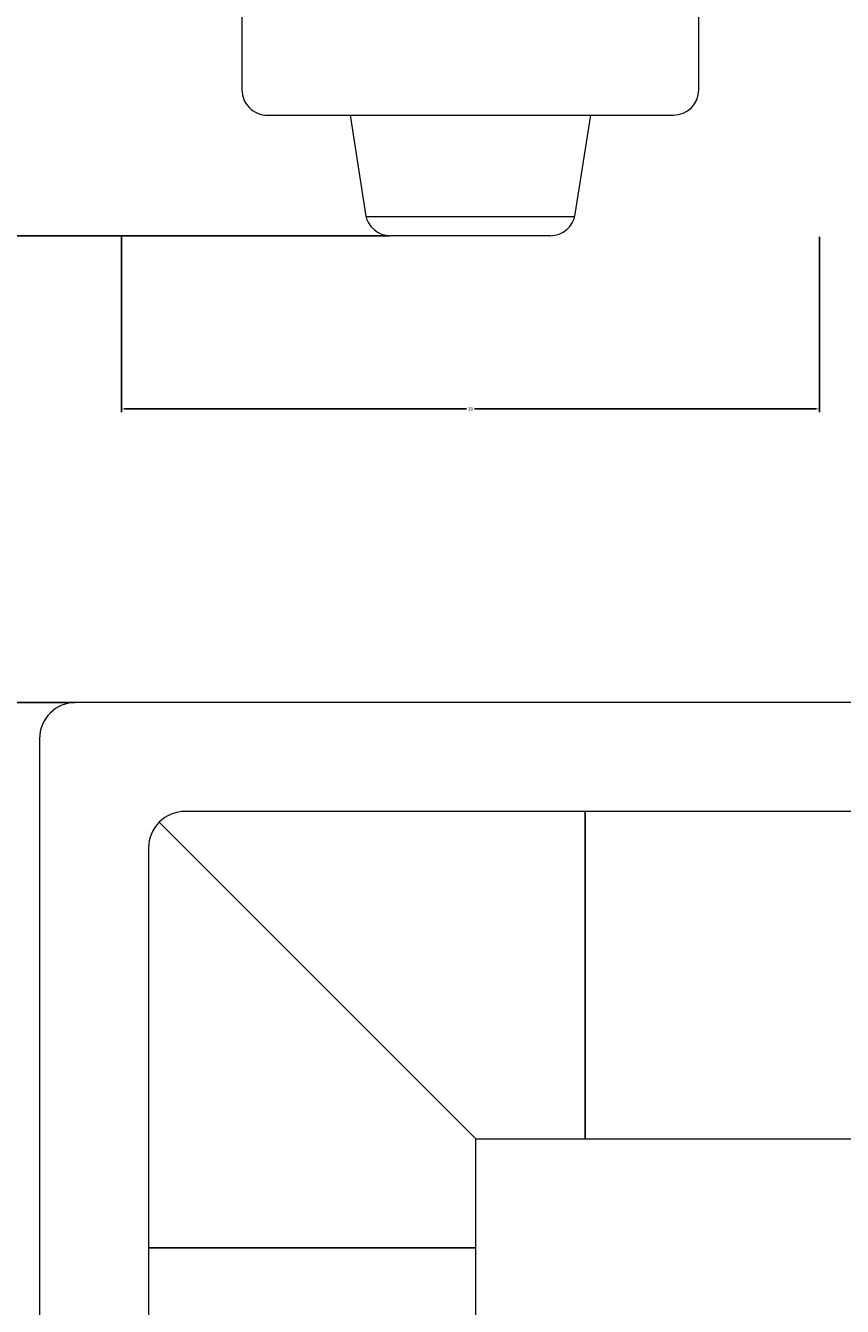
# Model space of a CAD drawing. Units: inches. Extents: x 2307 to 2544, y 2171 to 2540.
# Tile 5 of 52: x 2339 to 2384, y 2247 to 2317. Entities that reach past the tile are written whole.
import ezdxf

# ---------------------------------------------------------------- set-up
doc = ezdxf.new("R2010")
doc.units = ezdxf.units.IN
doc.layers.add('A-ANNO-DIMS', color=2, linetype='Continuous', lineweight=18)
doc.layers.add('A-FURN', color=8, linetype='Continuous', lineweight=18)
doc.styles.get("Standard").update_dxf_attribs({"font": 'arial.ttf'})
doc.dimstyles.get("Standard").update_dxf_attribs({"dimtxt": 0.18, "dimasz": 0.18, "dimexe": 0.18, "dimexo": 0.0625, "dimgap": 0.09, "dimtad": 0, "dimtih": 1, "dimtoh": 1, "dimdec": 4, "dimzin": 0, "dimdsep": 46, "dimtxsty": 'Standard', "dimcen": 0.09, "dimadec": 0, "dimazin": 0, "dimtfac": 1, "dimtdec": 4, "dimtofl": 0, "dimtmove": 0, "dimatfit": 3, "dimfxl": 1, "dimtolj": 1, "dimtzin": 0, "dimarcsym": 0})

# ---------------------------------------------------------------- blocks, each defined once
blk = doc.blocks.new('Dining Set - 36 x 72 in.')
for p, q in [((-20.29, 27.5), (-7.71, 27.5)), ((7.71, 27.5), (20.29, 27.5)), ((-22.26, 25.81), (-23.48, 18)), ((-22.23, 26), (-5.76, 26)), ((-4.52, 18), (-5.74, 25.81)), ((5.74, 25.81), (4.52, 18)), ((5.77, 26), (22.24, 26)), ((23.48, 18), (22.26, 25.81)), ((34, 18), (-34, 18)), ((-36, 16), (-36, -16)), ((36, -16), (36, 16)), ((-43.81, 8.26), (-36, 9.48)), ((43.81, 8.26), (36, 9.48)), ((-44, 8.23), (-44, -8.24)), ((44, 8.23), (44, -8.24)), ((-45.5, 6.29), (-45.5, -6.29)), ((45.5, 6.29), (45.5, -6.29)), ((-36, -9.48), (-43.81, -8.26)), ((36, -9.48), (43.81, -8.26)), ((-34, -18), (34, -18)), ((-22.26, -25.81), (-23.48, -18)), ((-4.52, -18), (-5.74, -25.81)), ((5.74, -25.81), (4.52, -18)), ((23.48, -18), (22.26, -25.81)), ((-22.23, -26), (-5.76, -26)), ((5.77, -26), (22.24, -26)), ((-20.29, -27.5), (-7.71, -27.5)), ((7.71, -27.5), (20.29, -27.5))]:
    blk.add_line(p, q)
for centre, start, end in [((-20.29, 25.5), 90, 171.1198), ((-7.71, 25.5), 8.881, 90), ((7.71, 25.5), 90, 171.1198), ((20.29, 25.5), 8.881, 90), ((-34, 16), 90, 180), ((34, 16), 0, 90), ((-43.5, 6.29), 98.8806, 180), ((43.5, 6.29), 0, 81.1194), ((-43.5, -6.29), 180, 261.1194), ((43.5, -6.29), 278.8806, 0), ((-34, -16), 180, 270), ((34, -16), 270, 0), ((-20.29, -25.5), 188.8802, 270), ((-7.71, -25.5), 270, 351.1191), ((7.71, -25.5), 188.8802, 270), ((20.29, -25.5), 270, 351.1191)]:
    blk.add_arc(centre, 2, start, end)
blk = doc.blocks.new('sofa')
for p, q in [((49, 6), (-19, 6)), ((-21, 4), (-21, -64)), ((-14.414, -0.586), (3, -18)), ((-15, -2), (-15, -60))]:
    blk.add_line(p, q)
blk.add_lwpolyline([(45, 0), (-13, 0, 0.414214), (-15, -2), (-15, -24), (3, -24), (3, -18)], format="xyb")
blk.add_lwpolyline([(3, -18), (9, -18), (9, 0), (-9, 0)])
for points in [[(27, 0), (9, 0), (9, -18), (27, -18)], [(3, -24), (-15, -24), (-15, -42), (3, -42)]]:
    blk.add_lwpolyline(points, close=True)
blk.add_arc((-19, 4), 2, 90, 180)
blk = doc.blocks.new('*D28')
at = {"layer": 'A-ANNO-DIMS', "color": 0, "lineweight": -2, "transparency": 16777216}
for p, q in [((2343.895, 2369.359), (2334.252, 2369.359)), ((2334.432, 2369.179), (2334.432, 2337.789)), ((2334.432, 2306.032), (2334.432, 2337.423)), ((2343.895, 2305.852), (2334.252, 2305.852))]:
    blk.add_line(p, q, dxfattribs=at)
at = {"layer": 'A-ANNO-DIMS', "color": 0, "transparency": 16777216}
for points in [[(2334.402, 2369.179), (2334.462, 2369.179), (2334.432, 2369.359)], [(2334.402, 2306.032), (2334.462, 2306.032), (2334.432, 2305.852)]]:
    blk.add_solid(points, dxfattribs=at)
at = {"layer": 'Defpoints', "color": 0, "transparency": 16777216}
for p in [(2343.958, 2369.359), (2334.432, 2305.852), (2343.958, 2305.852)]:
    blk.add_point(p, dxfattribs=at)
at = {"layer": 'A-ANNO-DIMS', "color": 0, "transparency": 16777216, "insert": (2334.432, 2337.606), "char_height": 0.18, "attachment_point": 5}
blk.add_mtext('\\A1;DINING SET 64', dxfattribs=at)
blk = doc.blocks.new('*D29')
at = {"layer": 'A-ANNO-DIMS', "color": 0, "lineweight": -2, "transparency": 16777216}
for p, q in [((2343.958, 2305.79), (2343.958, 2296.146)), ((2382.341, 2305.79), (2382.341, 2296.146)), ((2344.138, 2296.326), (2362.93, 2296.326)), ((2382.161, 2296.326), (2363.368, 2296.326))]:
    blk.add_line(p, q, dxfattribs=at)
at = {"layer": 'A-ANNO-DIMS', "color": 0, "transparency": 16777216}
for points in [[(2344.138, 2296.356), (2344.138, 2296.296), (2343.958, 2296.326)], [(2382.161, 2296.356), (2382.161, 2296.296), (2382.341, 2296.326)]]:
    blk.add_solid(points, dxfattribs=at)
at = {"layer": 'Defpoints', "color": 0, "transparency": 16777216}
for p in [(2343.958, 2305.852), (2382.341, 2305.852), (2382.341, 2296.326)]:
    blk.add_point(p, dxfattribs=at)
at = {"layer": 'A-ANNO-DIMS', "color": 0, "transparency": 16777216, "insert": (2363.149, 2296.326), "char_height": 0.18, "attachment_point": 5}
blk.add_mtext('\\A1;38', dxfattribs=at)
blk = doc.blocks.new('*D66')
at = {"layer": 'A-ANNO-DIMS', "color": 0, "lineweight": -2, "transparency": 16777216}
for p, q in [((2358.699, 2305.852), (2307.366, 2305.852)), ((2307.546, 2305.672), (2307.546, 2293.201)), ((2307.546, 2280.366), (2307.546, 2292.837)), ((2341.393, 2280.186), (2307.366, 2280.186))]:
    blk.add_line(p, q, dxfattribs=at)
at = {"layer": 'A-ANNO-DIMS', "color": 0, "transparency": 16777216}
for points in [[(2307.516, 2305.672), (2307.576, 2305.672), (2307.546, 2305.852)], [(2307.516, 2280.366), (2307.576, 2280.366), (2307.546, 2280.186)]]:
    blk.add_solid(points, dxfattribs=at)
at = {"layer": 'Defpoints', "color": 0, "transparency": 16777216}
for p in [(2307.546, 2305.852), (2358.761, 2305.852), (2341.456, 2280.186)]:
    blk.add_point(p, dxfattribs=at)
at = {"layer": 'A-ANNO-DIMS', "color": 0, "transparency": 16777216, "insert": (2307.546, 2293.019), "char_height": 0.18, "attachment_point": 5}
blk.add_mtext('\\A1;25.666', dxfattribs=at)

msp = doc.modelspace()

# ---------------------------------------------------------------- block references
at = {"layer": 'A-FURN', "xscale": 0.697875586402136, "yscale": 0.697875586402136, "zscale": 0.697875586402136, "rotation": 270}
msp.add_blockref('Dining Set - 36 x 72 in.', (2363.1494, 2337.6056), dxfattribs=at)
at = {"layer": 'A-FURN'}
msp.add_blockref('sofa', (2360.4557, 2274.1858), dxfattribs=at)

# ---------------------------------------------------------------- dimensions: what is measured, and where the dimension line sits
at = {"layer": 'A-ANNO-DIMS'}
dim = msp.add_linear_dim(base=(2334.4318, 2305.8523), p1=(2343.9578, 2369.3589), p2=(2343.9578, 2305.8523), angle=270, text='DINING SET <>', dimstyle='Standard', override={"dimdec": 0, "dimlfac": 1, "dimrnd": 0, "dimzin": 0, "dimdsep": 46, "dimlunit": 2}, dxfattribs=at)
dim.commit()
dim.dimension.update_dxf_attribs({"geometry": '*D28', "text_midpoint": (2334.4318, 2337.6056)})
dim = msp.add_linear_dim(base=(2307.54584, 2305.85226), p1=(2341.45575, 2280.18577), p2=(2358.76101, 2305.85226), angle=90, dimstyle='Standard', override={"dimdec": 3, "dimlfac": 1, "dimrnd": 0, "dimzin": 0, "dimdsep": 46, "dimlunit": 2}, dxfattribs=at)
dim.commit()
dim.dimension.update_dxf_attribs({"geometry": '*D66', "text_midpoint": (2307.54584, 2293.01902)})
dim = msp.add_linear_dim(base=(2382.341, 2296.3263), p1=(2343.9578, 2305.8523), p2=(2382.341, 2305.8523), dimstyle='Standard', override={"dimdec": 0, "dimlfac": 1, "dimrnd": 0, "dimzin": 0, "dimdsep": 46, "dimlunit": 2}, dxfattribs=at)
dim.commit()
dim.dimension.update_dxf_attribs({"geometry": '*D29', "text_midpoint": (2363.1494, 2296.3263)})

doc.saveas('drawing.dxf')
